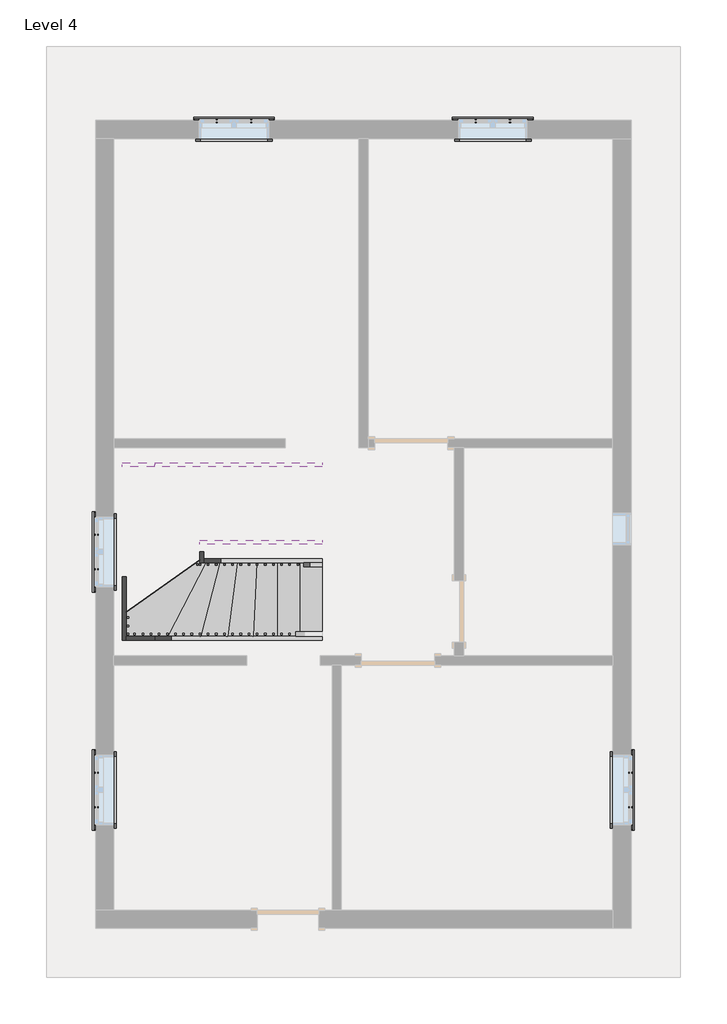
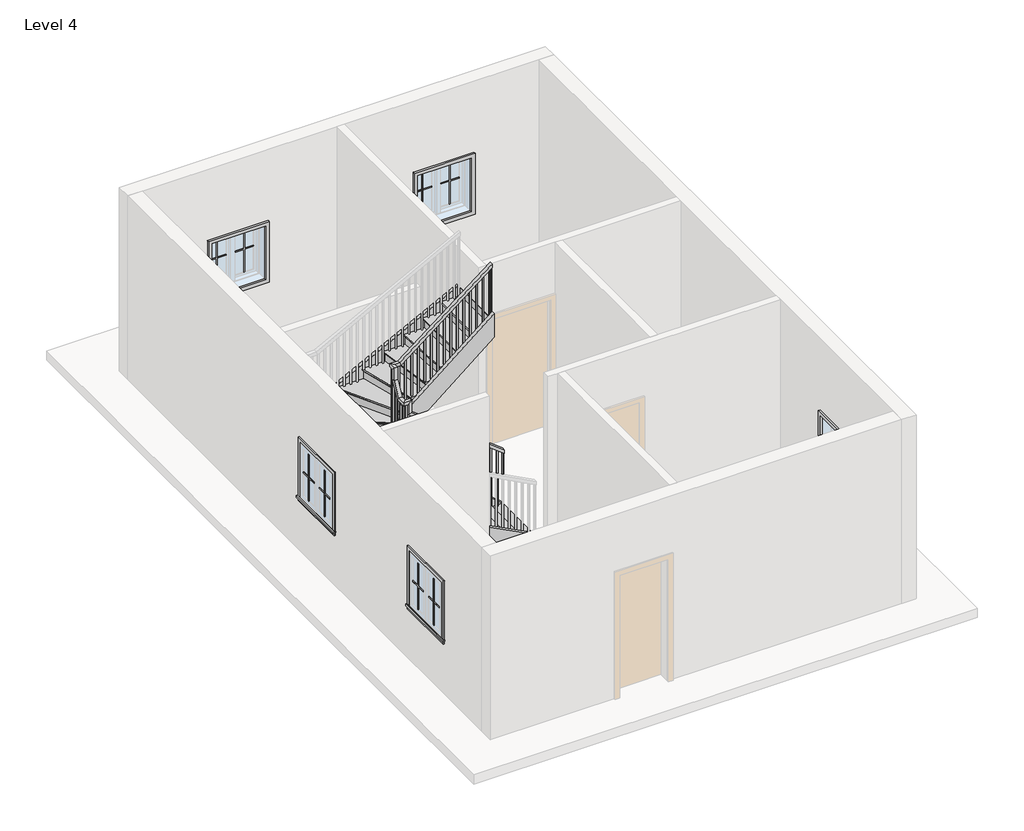
# One storey, part 2 of 2: 20 proxies, 8 members, 1 railing, 1 stair flight.
"""IFC4 building model written with IfcOpenShell, lengths in millimetres."""

from ifc_helpers import new_model, si_unit, frame, origin, place, context, project, spatial, polyline, outline, extrude, faceted_brep, transform, mapped, element, save
from components import muntin_pattern_2x2_muntin_pattern_2x2_b3fe6957, muntin_pattern_2x2_muntin_pattern_2x2_3e0ecaf2, trim_window_exterior_flat_with_sill_41619996, trim_window_interior_flat_picture_frame_51c85655, stair_flight_c61886c8

model = new_model("IFC4")

# Units and contexts
model_context = context("Model", 3, world=origin())
ifc_project = project(units=[si_unit("LENGTHUNIT", "METRE", prefix="MILLI")], contexts=[model_context])

# Site, building, storey
site = spatial("IfcSite", under=ifc_project)
building = spatial("IfcBuilding", under=site)
storey = spatial("IfcBuildingStorey", under=building, Name="Level 4", Elevation=6400.8)

# Proxies
placement = place(None, origin())
muntin_pattern_2x2_muntin_pattern_2x2_shape = muntin_pattern_2x2_muntin_pattern_2x2_b3fe6957(model_context)
element("IfcBuildingElementProxy", 1, Name="Muntin Pattern_2x2 : Muntin Pattern_2x2", ObjectType="Muntin Pattern_2x2 : Muntin Pattern_2x2", at=placement, inside=storey, context=model_context, shape_type="MappedRepresentation", body=[
    mapped(muntin_pattern_2x2_muntin_pattern_2x2_shape, transform((-3096.8324167, 5150.2179147, 7385.05), x_axis=(1.0, 0.0, 0.0), y_axis=(0.0, 1.0, 0.0), z_axis=(0.0, 0.0, 1.0))),
])
element("IfcBuildingElementProxy", 2, Name="Muntin Pattern_2x2 : Muntin Pattern_2x2", ObjectType="Muntin Pattern_2x2 : Muntin Pattern_2x2", at=placement, inside=storey, context=model_context, shape_type="MappedRepresentation", body=[
    mapped(muntin_pattern_2x2_muntin_pattern_2x2_shape, transform((122.6175833, 5150.2179147, 7385.05), x_axis=(1.0, 0.0, 0.0), y_axis=(0.0, 1.0, 0.0), z_axis=(0.0, 0.0, 1.0))),
])
element("IfcBuildingElementProxy", 3, Name="Muntin Pattern_2x2 : Muntin Pattern_2x2", ObjectType="Muntin Pattern_2x2 : Muntin Pattern_2x2", at=placement, inside=storey, context=model_context, shape_type="MappedRepresentation", body=[
    mapped(muntin_pattern_2x2_muntin_pattern_2x2_shape, transform((2051.4300833, -2960.3195853, 7385.05), x_axis=(0.0, -1.0, 0.0), y_axis=(1.0, 0.0, 0.0), z_axis=(0.0, 0.0, 1.0))),
])
element("IfcBuildingElementProxy", 4, Name="Muntin Pattern_2x2 : Muntin Pattern_2x2", ObjectType="Muntin Pattern_2x2 : Muntin Pattern_2x2", at=placement, inside=storey, context=model_context, shape_type="MappedRepresentation", body=[
    mapped(muntin_pattern_2x2_muntin_pattern_2x2_shape, transform((-4597.0199167, -3388.9445853, 7385.05), x_axis=(0.0, 1.0, 0.0), y_axis=(-1.0, 0.0, 0.0), z_axis=(0.0, 0.0, 1.0))),
])
element("IfcBuildingElementProxy", 5, Name="Muntin Pattern_2x2 : Muntin Pattern_2x2", ObjectType="Muntin Pattern_2x2 : Muntin Pattern_2x2", at=placement, inside=storey, context=model_context, shape_type="MappedRepresentation", body=[
    mapped(muntin_pattern_2x2_muntin_pattern_2x2_shape, transform((-4597.0199167, -426.6695853, 7385.05), x_axis=(0.0, 1.0, 0.0), y_axis=(-1.0, 0.0, 0.0), z_axis=(0.0, 0.0, 1.0))),
])
muntin_pattern_2x2_muntin_pattern_2x2_2_shape = muntin_pattern_2x2_muntin_pattern_2x2_3e0ecaf2(model_context)
element("IfcBuildingElementProxy", 6, Name="Muntin Pattern_2x2 : Muntin Pattern_2x2", ObjectType="Muntin Pattern_2x2 : Muntin Pattern_2x2", at=placement, inside=storey, context=model_context, shape_type="MappedRepresentation", body=[
    mapped(muntin_pattern_2x2_muntin_pattern_2x2_2_shape, transform((-2668.2074167, 5150.2179147, 7385.05), x_axis=(-1.0, 0.0, 0.0), y_axis=(0.0, -1.0, 0.0), z_axis=(0.0, 0.0, 1.0))),
])
element("IfcBuildingElementProxy", 7, Name="Muntin Pattern_2x2 : Muntin Pattern_2x2", ObjectType="Muntin Pattern_2x2 : Muntin Pattern_2x2", at=placement, inside=storey, context=model_context, shape_type="MappedRepresentation", body=[
    mapped(muntin_pattern_2x2_muntin_pattern_2x2_2_shape, transform((551.2425833, 5150.2179147, 7385.05), x_axis=(-1.0, 0.0, 0.0), y_axis=(0.0, -1.0, 0.0), z_axis=(0.0, 0.0, 1.0))),
])
element("IfcBuildingElementProxy", 8, Name="Muntin Pattern_2x2 : Muntin Pattern_2x2", ObjectType="Muntin Pattern_2x2 : Muntin Pattern_2x2", at=placement, inside=storey, context=model_context, shape_type="MappedRepresentation", body=[
    mapped(muntin_pattern_2x2_muntin_pattern_2x2_2_shape, transform((2051.4300833, -3388.9445853, 7385.05), x_axis=(0.0, 1.0, 0.0), y_axis=(-1.0, 0.0, 0.0), z_axis=(0.0, 0.0, 1.0))),
])
element("IfcBuildingElementProxy", 9, Name="Muntin Pattern_2x2 : Muntin Pattern_2x2", ObjectType="Muntin Pattern_2x2 : Muntin Pattern_2x2", at=placement, inside=storey, context=model_context, shape_type="MappedRepresentation", body=[
    mapped(muntin_pattern_2x2_muntin_pattern_2x2_2_shape, transform((-4597.0199167, -2960.3195853, 7385.05), x_axis=(0.0, -1.0, 0.0), y_axis=(1.0, 0.0, 0.0), z_axis=(0.0, 0.0, 1.0))),
])
element("IfcBuildingElementProxy", 10, Name="Muntin Pattern_2x2 : Muntin Pattern_2x2", ObjectType="Muntin Pattern_2x2 : Muntin Pattern_2x2", at=placement, inside=storey, context=model_context, shape_type="MappedRepresentation", body=[
    mapped(muntin_pattern_2x2_muntin_pattern_2x2_2_shape, transform((-4597.0199167, 1.9554147, 7385.05), x_axis=(0.0, -1.0, 0.0), y_axis=(1.0, 0.0, 0.0), z_axis=(0.0, 0.0, 1.0))),
])
trim_window_exterior_flat_with_sill_shape = trim_window_exterior_flat_with_sill_41619996(model_context)
element("IfcBuildingElementProxy", 11, Name="Trim-Window-Exterior-Flat : with Sill", ObjectType="Trim-Window-Exterior-Flat : with Sill", at=placement, inside=storey, context=model_context, shape_type="MappedRepresentation", body=[
    mapped(trim_window_exterior_flat_with_sill_shape, transform((-2882.5199167, 5159.7429147, 8229.6), x_axis=(-1.0, 0.0, 0.0), y_axis=(0.0, 0.0, 1.0), z_axis=(0.0, 1.0, 0.0))),
])
element("IfcBuildingElementProxy", 12, Name="Trim-Window-Exterior-Flat : with Sill", ObjectType="Trim-Window-Exterior-Flat : with Sill", at=placement, inside=storey, context=model_context, shape_type="MappedRepresentation", body=[
    mapped(trim_window_exterior_flat_with_sill_shape, transform((336.9300833, 5159.7429147, 8229.6), x_axis=(-1.0, 0.0, 0.0), y_axis=(0.0, 0.0, 1.0), z_axis=(0.0, 1.0, 0.0))),
])
element("IfcBuildingElementProxy", 13, Name="Trim-Window-Exterior-Flat : with Sill", ObjectType="Trim-Window-Exterior-Flat : with Sill", at=placement, inside=storey, context=model_context, shape_type="MappedRepresentation", body=[
    mapped(trim_window_exterior_flat_with_sill_shape, transform((2060.9550833, -3174.6320853, 8229.6), x_axis=(0.0, 1.0, 0.0), y_axis=(0.0, 0.0, 1.0), z_axis=(1.0, 0.0, 0.0))),
])
element("IfcBuildingElementProxy", 14, Name="Trim-Window-Exterior-Flat : with Sill", ObjectType="Trim-Window-Exterior-Flat : with Sill", at=placement, inside=storey, context=model_context, shape_type="MappedRepresentation", body=[
    mapped(trim_window_exterior_flat_with_sill_shape, transform((-4606.5449167, -3174.6320853, 8229.6), x_axis=(0.0, -1.0, 0.0), y_axis=(0.0, 0.0, 1.0), z_axis=(-1.0, 0.0, 0.0))),
])
element("IfcBuildingElementProxy", 15, Name="Trim-Window-Exterior-Flat : with Sill", ObjectType="Trim-Window-Exterior-Flat : with Sill", at=placement, inside=storey, context=model_context, shape_type="MappedRepresentation", body=[
    mapped(trim_window_exterior_flat_with_sill_shape, transform((-4606.5449167, -212.3570853, 8229.6), x_axis=(0.0, -1.0, 0.0), y_axis=(0.0, 0.0, 1.0), z_axis=(-1.0, 0.0, 0.0))),
])
trim_window_interior_flat_picture_frame_shape = trim_window_interior_flat_picture_frame_51c85655(model_context)
element("IfcBuildingElementProxy", 16, Name="Trim-Window-Interior-Flat : Picture Frame", ObjectType="Trim-Window-Interior-Flat : Picture Frame", at=placement, inside=storey, context=model_context, shape_type="MappedRepresentation", body=[
    mapped(trim_window_interior_flat_picture_frame_shape, transform((-2882.5199167, 4931.1429147, 8229.6), x_axis=(1.0, 0.0, 0.0), y_axis=(0.0, 0.0, 1.0), z_axis=(0.0, -1.0, 0.0))),
])
element("IfcBuildingElementProxy", 17, Name="Trim-Window-Interior-Flat : Picture Frame", ObjectType="Trim-Window-Interior-Flat : Picture Frame", at=placement, inside=storey, context=model_context, shape_type="MappedRepresentation", body=[
    mapped(trim_window_interior_flat_picture_frame_shape, transform((336.9300833, 4931.1429147, 8229.6), x_axis=(1.0, 0.0, 0.0), y_axis=(0.0, 0.0, 1.0), z_axis=(0.0, -1.0, 0.0))),
])
element("IfcBuildingElementProxy", 18, Name="Trim-Window-Interior-Flat : Picture Frame", ObjectType="Trim-Window-Interior-Flat : Picture Frame", at=placement, inside=storey, context=model_context, shape_type="MappedRepresentation", body=[
    mapped(trim_window_interior_flat_picture_frame_shape, transform((1832.3550833, -3174.6320853, 8229.6), x_axis=(0.0, -1.0, 0.0), y_axis=(0.0, 0.0, 1.0), z_axis=(-1.0, 0.0, 0.0))),
])
element("IfcBuildingElementProxy", 19, Name="Trim-Window-Interior-Flat : Picture Frame", ObjectType="Trim-Window-Interior-Flat : Picture Frame", at=placement, inside=storey, context=model_context, shape_type="MappedRepresentation", body=[
    mapped(trim_window_interior_flat_picture_frame_shape, transform((-4377.9449167, -3174.6320853, 8229.6), x_axis=(0.0, 1.0, 0.0), y_axis=(0.0, 0.0, 1.0), z_axis=(1.0, 0.0, 0.0))),
])
element("IfcBuildingElementProxy", 20, Name="Trim-Window-Interior-Flat : Picture Frame", ObjectType="Trim-Window-Interior-Flat : Picture Frame", at=placement, inside=storey, context=model_context, shape_type="MappedRepresentation", body=[
    mapped(trim_window_interior_flat_picture_frame_shape, transform((-4377.9449167, -212.3570853, 8229.6), x_axis=(0.0, 1.0, 0.0), y_axis=(0.0, 0.0, 1.0), z_axis=(1.0, 0.0, 0.0))),
])

# Members
element("IfcMember", 21, ObjectType="Stringer - 2\" Width", at=placement, inside=storey, context=model_context, shape_type="SweptSolid", body=[
    extrude(outline(polyline([(6400.8, -1783.4132248), (6630.439954, -1783.4132248), (7706.1956453, -3870.8304165), (7363.300629, -3870.8304165), (6400.8, -2003.1755424), (6400.8, -1783.4132248)])), frame((0.0, -1310.9070853, 0.0), z_axis=(0.0, 1.0, 0.0), x_axis=(0.0, 0.0, 1.0)), (0.0, 0.0, 1.0), 50.8),
])
element("IfcMember", 22, ObjectType="Stringer - 2\" Width", at=placement, inside=storey, context=model_context, shape_type="SweptSolid", body=[
    extrude(outline(polyline([(-3870.8304165, -1260.1070853), (-3870.8304165, -1310.9070853), (-4225.5449167, -1310.9070853), (-4225.5449167, -1260.1070853), (-3870.8304165, -1260.1070853)])), frame((0.0, 0.0, 7363.300629), z_axis=(0.0, 0.0, 1.0), x_axis=(1.0, 0.0, 0.0)), (0.0, 0.0, 1.0), 342.8950162),
])
element("IfcMember", 23, ObjectType="Stringer - 2\" Width", at=placement, inside=storey, context=model_context, shape_type="SweptSolid", body=[
    extrude(outline(polyline([(-1310.9070853, 7401.3956453), (-1310.9070853, 7689.8952212), (811.1127974, 8370.7972697), (848.0929147, 8370.7972697), (848.0929147, 8039.7682298), (-1141.3846024, 7401.3956453), (-1310.9070853, 7401.3956453)])), frame((-4276.3449167, 0.0, 0.0), z_axis=(1.0, 0.0, 0.0), x_axis=(0.0, 1.0, 0.0)), (0.0, 0.0, 1.0), 50.8),
])
element("IfcMember", 24, ObjectType="Stringer - 2\" Width", at=placement, inside=storey, context=model_context, shape_type="SweptSolid", body=[
    extrude(outline(polyline([(-4276.3449167, 848.0929147), (-4276.3449167, 898.8929147), (-3870.8304165, 898.8929147), (-3870.8304165, 848.0929147), (-4276.3449167, 848.0929147)])), frame((0.0, 0.0, 8050.6904473), z_axis=(0.0, 0.0, 1.0), x_axis=(1.0, 0.0, 0.0)), (0.0, 0.0, 1.0), 320.1068224),
])
element("IfcMember", 25, ObjectType="Stringer - 2\" Width", at=placement, inside=storey, context=model_context, shape_type="SweptSolid", body=[
    extrude(outline(polyline([(8370.7972697, -3870.8304165), (8050.6904473, -3870.8304165), (9126.4461385, -1783.4132248), (9446.5529609, -1783.4132248), (8370.7972697, -3870.8304165)])), frame((0.0, 848.0929147, 0.0), z_axis=(0.0, 1.0, 0.0), x_axis=(0.0, 0.0, 1.0)), (0.0, 0.0, 1.0), 50.8),
])
element("IfcMember", 26, ObjectType="Stringer - 2\" Width", at=placement, inside=storey, context=model_context, shape_type="SweptSolid", body=[
    extrude(outline(polyline([(6400.8, -1783.4132248), (6576.9764461, -1783.4132248), (7781.218648, -3260.3449167), (7387.9410923, -3260.3449167), (6400.8, -2049.6748694), (6400.8, -1783.4132248)])), frame((0.0, -345.7070853, 0.0), z_axis=(0.0, 1.0, 0.0), x_axis=(0.0, 0.0, 1.0)), (0.0, 0.0, 1.0), 50.8),
])
element("IfcMember", 27, ObjectType="Stringer - 2\" Width", at=placement, inside=storey, context=model_context, shape_type="SweptSolid", body=[
    extrude(outline(polyline([(-345.7070853, 7429.3617647), (-345.7070853, 7974.0682978), (-139.0699679, 8326.9409689), (-117.1070853, 8326.9409689), (-117.1070853, 7761.265107), (-311.464868, 7429.3617647), (-345.7070853, 7429.3617647)])), frame((-3311.1449167, 0.0, 0.0), z_axis=(1.0, 0.0, 0.0), x_axis=(0.0, 1.0, 0.0)), (0.0, 0.0, 1.0), 50.8),
])
element("IfcMember", 28, ObjectType="Stringer - 2\" Width", at=placement, inside=storey, context=model_context, shape_type="SweptSolid", body=[
    extrude(outline(polyline([(8326.9409689, -3311.1449167), (7933.6634131, -3311.1449167), (9179.3262875, -1783.4132248), (9572.6038432, -1783.4132248), (8326.9409689, -3311.1449167)])), frame((0.0, -117.1070853, 0.0), z_axis=(0.0, 1.0, 0.0), x_axis=(0.0, 0.0, 1.0)), (0.0, 0.0, 1.0), 50.8),
])

# Railing
element("IfcRailing", 29, ObjectType="Handrail - Rectangular", at=placement, inside=storey, context=model_context, shape_type="SolidModel", body=[
    faceted_brep([(-1783.4132248, -396.5070853, 7484.5333333), (-1783.4132248, -396.5070853, 7420.2000346), (-1783.4132248, -345.7070853, 7420.2000346), (-1783.4132248, -345.7070853, 7484.5333333), (-3234.9449167, -396.5070853, 8612.4191036), (-3285.7449167, -396.5070853, 8587.5590024), (-3285.7449167, -345.7070853, 8587.5590024), (-3234.9449167, -345.7070853, 8612.4191036), (-3234.9449167, -396.5070853, 8815.4281882), (-3285.7449167, -396.5070853, 8764.6281882), (-3285.7449167, -345.7070853, 8764.6281882), (-3234.9449167, -345.7070853, 8815.4281882), (-3361.9449167, -396.5070853, 8815.4281882), (-3361.9449167, -396.5070853, 8764.6281882), (-3311.1449167, -345.7070853, 8764.6281882), (-3311.1449167, -345.7070853, 8815.4281882), (-3361.9449167, -269.5070853, 8815.4281882), (-3361.9449167, -240.3857515, 8764.6281882), (-3311.1449167, -240.3857515, 8764.6281882), (-3311.1449167, -269.5070853, 8815.4281882), (-3361.9449167, -142.5070853, 9032.3051451), (-3361.9449167, -91.7070853, 9018.5256424), (-3311.1449167, -91.7070853, 9018.5256424), (-3311.1449167, -142.5070853, 9032.3051451), (-3361.9449167, -142.5070853, 9235.3142297), (-3361.9449167, -91.7070853, 9184.5142297), (-3311.1449167, -91.7070853, 9184.5142297), (-3311.1449167, -142.5070853, 9235.3142297), (-3361.9449167, -15.5070853, 9235.3142297), (-3361.9449167, -15.5070853, 9184.5142297), (-3311.1449167, -66.3070853, 9184.5142297), (-3311.1449167, -66.3070853, 9235.3142297), (-3234.9449167, -15.5070853, 9235.3142297), (-3217.5282487, -15.5070853, 9184.5142297), (-3217.5282487, -66.3070853, 9184.5142297), (-3234.9449167, -66.3070853, 9235.3142297), (-1783.4132248, -15.5070853, 10363.2), (-1783.4132248, -66.3070853, 10363.2), (-1783.4132248, -66.3070853, 10298.8667013), (-1783.4132248, -15.5070853, 10298.8667013)], [[[0, 1, 2, 3]], [[1, 0, 4, 5]], [[2, 1, 5, 6]], [[3, 2, 6, 7]], [[0, 3, 7, 4]], [[5, 4, 8, 9]], [[6, 5, 9, 10]], [[7, 6, 10, 11]], [[4, 7, 11, 8]], [[9, 8, 12, 13]], [[10, 9, 13, 14]], [[11, 10, 14, 15]], [[8, 11, 15, 12]], [[13, 12, 16, 17]], [[14, 13, 17, 18]], [[15, 14, 18, 19]], [[12, 15, 19, 16]], [[17, 16, 20, 21]], [[18, 17, 21, 22]], [[19, 18, 22, 23]], [[16, 19, 23, 20]], [[21, 20, 24, 25]], [[22, 21, 25, 26]], [[23, 22, 26, 27]], [[20, 23, 27, 24]], [[25, 24, 28, 29]], [[26, 25, 29, 30]], [[27, 26, 30, 31]], [[24, 27, 31, 28]], [[29, 28, 32, 33]], [[30, 29, 33, 34]], [[31, 30, 34, 35]], [[28, 31, 35, 32]], [[36, 37, 38, 39]], [[33, 32, 36, 39]], [[34, 33, 39, 38]], [[35, 34, 38, 37]], [[32, 35, 37, 36]]]),
    extrude(outline(polyline([(10283.6316852, -1803.0199167), (10268.8292361, -1822.0699167), (9279.4666667, -1822.0699167), (9279.4666667, -1803.0199167), (10283.6316852, -1803.0199167)])), frame((0.0, -50.4320853, 0.0), z_axis=(0.0, 1.0, 0.0), x_axis=(0.0, 0.0, 1.0)), (0.0, 0.0, 1.0), 19.05),
    extrude(outline(polyline([(10204.6852902, -1904.6199167), (10189.8828411, -1923.6699167), (9279.4666667, -1923.6699167), (9279.4666667, -1904.6199167), (10204.6852902, -1904.6199167)])), frame((0.0, -50.4320853, 0.0), z_axis=(0.0, 1.0, 0.0), x_axis=(0.0, 0.0, 1.0)), (0.0, 0.0, 1.0), 19.05),
    extrude(outline(polyline([(10125.7388952, -2006.2199167), (10110.9364462, -2025.2699167), (9279.4666667, -2025.2699167), (9279.4666667, -2006.2199167), (10125.7388952, -2006.2199167)])), frame((0.0, -50.4320853, 0.0), z_axis=(0.0, 1.0, 0.0), x_axis=(0.0, 0.0, 1.0)), (0.0, 0.0, 1.0), 19.05),
    extrude(outline(polyline([(10046.7925003, -2107.8199167), (10031.9900512, -2126.8699167), (9110.1333333, -2126.8699167), (9110.1333333, -2107.8199167), (10046.7925003, -2107.8199167)])), frame((0.0, -50.4320853, 0.0), z_axis=(0.0, 1.0, 0.0), x_axis=(0.0, 0.0, 1.0)), (0.0, 0.0, 1.0), 19.05),
    extrude(outline(polyline([(9967.8461053, -2209.4199167), (9953.0436562, -2228.4699167), (9110.1333333, -2228.4699167), (9110.1333333, -2209.4199167), (9967.8461053, -2209.4199167)])), frame((0.0, -50.4320853, 0.0), z_axis=(0.0, 1.0, 0.0), x_axis=(0.0, 0.0, 1.0)), (0.0, 0.0, 1.0), 19.05),
    extrude(outline(polyline([(9888.8997103, -2311.0199167), (9874.0972613, -2330.0699167), (9110.1333333, -2330.0699167), (9110.1333333, -2311.0199167), (9888.8997103, -2311.0199167)])), frame((0.0, -50.4320853, 0.0), z_axis=(0.0, 1.0, 0.0), x_axis=(0.0, 0.0, 1.0)), (0.0, 0.0, 1.0), 19.05),
    extrude(outline(polyline([(9809.9533154, -2412.6199167), (9795.1508663, -2431.6699167), (8940.8, -2431.6699167), (8940.8, -2412.6199167), (9809.9533154, -2412.6199167)])), frame((0.0, -50.4320853, 0.0), z_axis=(0.0, 1.0, 0.0), x_axis=(0.0, 0.0, 1.0)), (0.0, 0.0, 1.0), 19.05),
    extrude(outline(polyline([(9731.0069204, -2514.2199167), (9716.2044713, -2533.2699167), (8940.8, -2533.2699167), (8940.8, -2514.2199167), (9731.0069204, -2514.2199167)])), frame((0.0, -50.4320853, 0.0), z_axis=(0.0, 1.0, 0.0), x_axis=(0.0, 0.0, 1.0)), (0.0, 0.0, 1.0), 19.05),
    extrude(outline(polyline([(9652.0605254, -2615.8199167), (9637.2580764, -2634.8699167), (8771.4666667, -2634.8699167), (8771.4666667, -2615.8199167), (9652.0605254, -2615.8199167)])), frame((0.0, -50.4320853, 0.0), z_axis=(0.0, 1.0, 0.0), x_axis=(0.0, 0.0, 1.0)), (0.0, 0.0, 1.0), 19.05),
    extrude(outline(polyline([(9573.1141304, -2717.4199167), (9558.3116814, -2736.4699167), (8771.4666667, -2736.4699167), (8771.4666667, -2717.4199167), (9573.1141304, -2717.4199167)])), frame((0.0, -50.4320853, 0.0), z_axis=(0.0, 1.0, 0.0), x_axis=(0.0, 0.0, 1.0)), (0.0, 0.0, 1.0), 19.05),
    extrude(outline(polyline([(9494.1677355, -2819.0199167), (9479.3652864, -2838.0699167), (8771.4666667, -2838.0699167), (8771.4666667, -2819.0199167), (9494.1677355, -2819.0199167)])), frame((0.0, -50.4320853, 0.0), z_axis=(0.0, 1.0, 0.0), x_axis=(0.0, 0.0, 1.0)), (0.0, 0.0, 1.0), 19.05),
    extrude(outline(polyline([(9415.2213405, -2920.6199167), (9400.4188914, -2939.6699167), (8602.1333333, -2939.6699167), (8602.1333333, -2920.6199167), (9415.2213405, -2920.6199167)])), frame((0.0, -50.4320853, 0.0), z_axis=(0.0, 1.0, 0.0), x_axis=(0.0, 0.0, 1.0)), (0.0, 0.0, 1.0), 19.05),
    extrude(outline(polyline([(9336.2749455, -3022.2199167), (9321.4724965, -3041.2699167), (8602.1333333, -3041.2699167), (8602.1333333, -3022.2199167), (9336.2749455, -3022.2199167)])), frame((0.0, -50.4320853, 0.0), z_axis=(0.0, 1.0, 0.0), x_axis=(0.0, 0.0, 1.0)), (0.0, 0.0, 1.0), 19.05),
    extrude(outline(polyline([(9257.3285506, -3123.8199167), (9242.5261015, -3142.8699167), (8432.8, -3142.8699167), (8432.8, -3123.8199167), (9257.3285506, -3123.8199167)])), frame((0.0, -50.4320853, 0.0), z_axis=(0.0, 1.0, 0.0), x_axis=(0.0, 0.0, 1.0)), (0.0, 0.0, 1.0), 19.05),
    extrude(outline(polyline([(9178.3821556, -3225.4199167), (9163.5797065, -3244.4699167), (8432.8, -3244.4699167), (8432.8, -3225.4199167), (9178.3821556, -3225.4199167)])), frame((0.0, -50.4320853, 0.0), z_axis=(0.0, 1.0, 0.0), x_axis=(0.0, 0.0, 1.0)), (0.0, 0.0, 1.0), 19.05),
    extrude(outline(polyline([(-3327.0199167, -75.8320853), (-3346.0699167, -75.8320853), (-3346.0699167, -56.7820853), (-3327.0199167, -56.7820853), (-3327.0199167, -75.8320853)])), frame((0.0, 0.0, 8094.1333333), z_axis=(0.0, 0.0, 1.0), x_axis=(1.0, 0.0, 0.0)), (0.0, 0.0, 1.0), 1090.3808964),
    extrude(outline(polyline([(-177.4320853, 8872.1336964), (-158.3820853, 8904.66524), (-158.3820853, 7924.8), (-177.4320853, 7924.8), (-177.4320853, 8872.1336964)])), frame((-3346.0699167, 0.0, 0.0), z_axis=(1.0, 0.0, 0.0), x_axis=(0.0, 1.0, 0.0)), (0.0, 0.0, 1.0), 19.05),
    extrude(outline(polyline([(-279.0320853, 8698.6321309), (-259.9820853, 8731.1636744), (-259.9820853, 7755.4666667), (-279.0320853, 7755.4666667), (-279.0320853, 8698.6321309)])), frame((-3346.0699167, 0.0, 0.0), z_axis=(1.0, 0.0, 0.0), x_axis=(0.0, 1.0, 0.0)), (0.0, 0.0, 1.0), 19.05),
    extrude(outline(polyline([(-3297.8882248, -361.5820853), (-3297.8882248, -380.6320853), (-3316.9382248, -380.6320853), (-3316.9382248, -361.5820853), (-3297.8882248, -361.5820853)])), frame((0.0, 0.0, 7586.1333333), z_axis=(0.0, 0.0, 1.0), x_axis=(1.0, 0.0, 0.0)), (0.0, 0.0, 1.0), 1178.4948549),
    extrude(outline(polyline([(8518.0483397, -3196.2882248), (8532.8507888, -3215.3382248), (7416.8, -3215.3382248), (7416.8, -3196.2882248), (8518.0483397, -3196.2882248)])), frame((0.0, -380.6320853, 0.0), z_axis=(0.0, 1.0, 0.0), x_axis=(0.0, 0.0, 1.0)), (0.0, 0.0, 1.0), 19.05),
    extrude(outline(polyline([(8439.1019447, -3094.6882248), (8453.9043938, -3113.7382248), (7416.8, -3113.7382248), (7416.8, -3094.6882248), (8439.1019447, -3094.6882248)])), frame((0.0, -380.6320853, 0.0), z_axis=(0.0, 1.0, 0.0), x_axis=(0.0, 0.0, 1.0)), (0.0, 0.0, 1.0), 19.05),
    extrude(outline(polyline([(8360.1555498, -2993.0882248), (8374.9579988, -3012.1382248), (7247.4666667, -3012.1382248), (7247.4666667, -2993.0882248), (8360.1555498, -2993.0882248)])), frame((0.0, -380.6320853, 0.0), z_axis=(0.0, 1.0, 0.0), x_axis=(0.0, 0.0, 1.0)), (0.0, 0.0, 1.0), 19.05),
    extrude(outline(polyline([(8281.2091548, -2891.4882248), (8296.0116039, -2910.5382248), (7247.4666667, -2910.5382248), (7247.4666667, -2891.4882248), (8281.2091548, -2891.4882248)])), frame((0.0, -380.6320853, 0.0), z_axis=(0.0, 1.0, 0.0), x_axis=(0.0, 0.0, 1.0)), (0.0, 0.0, 1.0), 19.05),
    extrude(outline(polyline([(8202.2627598, -2789.8882248), (8217.0652089, -2808.9382248), (7078.1333333, -2808.9382248), (7078.1333333, -2789.8882248), (8202.2627598, -2789.8882248)])), frame((0.0, -380.6320853, 0.0), z_axis=(0.0, 1.0, 0.0), x_axis=(0.0, 0.0, 1.0)), (0.0, 0.0, 1.0), 19.05),
    extrude(outline(polyline([(8123.3163649, -2688.2882248), (8138.1188139, -2707.3382248), (7078.1333333, -2707.3382248), (7078.1333333, -2688.2882248), (8123.3163649, -2688.2882248)])), frame((0.0, -380.6320853, 0.0), z_axis=(0.0, 1.0, 0.0), x_axis=(0.0, 0.0, 1.0)), (0.0, 0.0, 1.0), 19.05),
    extrude(outline(polyline([(8044.3699699, -2586.6882248), (8059.1724189, -2605.7382248), (6908.8, -2605.7382248), (6908.8, -2586.6882248), (8044.3699699, -2586.6882248)])), frame((0.0, -380.6320853, 0.0), z_axis=(0.0, 1.0, 0.0), x_axis=(0.0, 0.0, 1.0)), (0.0, 0.0, 1.0), 19.05),
    extrude(outline(polyline([(7965.4235749, -2485.0882248), (7980.226024, -2504.1382248), (6908.8, -2504.1382248), (6908.8, -2485.0882248), (7965.4235749, -2485.0882248)])), frame((0.0, -380.6320853, 0.0), z_axis=(0.0, 1.0, 0.0), x_axis=(0.0, 0.0, 1.0)), (0.0, 0.0, 1.0), 19.05),
    extrude(outline(polyline([(7886.4771799, -2383.4882248), (7901.279629, -2402.5382248), (6908.8, -2402.5382248), (6908.8, -2383.4882248), (7886.4771799, -2383.4882248)])), frame((0.0, -380.6320853, 0.0), z_axis=(0.0, 1.0, 0.0), x_axis=(0.0, 0.0, 1.0)), (0.0, 0.0, 1.0), 19.05),
    extrude(outline(polyline([(7807.530785, -2281.8882248), (7822.333234, -2300.9382248), (6739.4666667, -2300.9382248), (6739.4666667, -2281.8882248), (7807.530785, -2281.8882248)])), frame((0.0, -380.6320853, 0.0), z_axis=(0.0, 1.0, 0.0), x_axis=(0.0, 0.0, 1.0)), (0.0, 0.0, 1.0), 19.05),
    extrude(outline(polyline([(7728.58439, -2180.2882248), (7743.3868391, -2199.3382248), (6739.4666667, -2199.3382248), (6739.4666667, -2180.2882248), (7728.58439, -2180.2882248)])), frame((0.0, -380.6320853, 0.0), z_axis=(0.0, 1.0, 0.0), x_axis=(0.0, 0.0, 1.0)), (0.0, 0.0, 1.0), 19.05),
    extrude(outline(polyline([(7649.637995, -2078.6882248), (7664.4404441, -2097.7382248), (6739.4666667, -2097.7382248), (6739.4666667, -2078.6882248), (7649.637995, -2078.6882248)])), frame((0.0, -380.6320853, 0.0), z_axis=(0.0, 1.0, 0.0), x_axis=(0.0, 0.0, 1.0)), (0.0, 0.0, 1.0), 19.05),
    extrude(outline(polyline([(7570.6916001, -1977.0882248), (7585.4940491, -1996.1382248), (6570.1333333, -1996.1382248), (6570.1333333, -1977.0882248), (7570.6916001, -1977.0882248)])), frame((0.0, -380.6320853, 0.0), z_axis=(0.0, 1.0, 0.0), x_axis=(0.0, 0.0, 1.0)), (0.0, 0.0, 1.0), 19.05),
    extrude(outline(polyline([(7491.7452051, -1875.4882248), (7506.5476541, -1894.5382248), (6570.1333333, -1894.5382248), (6570.1333333, -1875.4882248), (7491.7452051, -1875.4882248)])), frame((0.0, -380.6320853, 0.0), z_axis=(0.0, 1.0, 0.0), x_axis=(0.0, 0.0, 1.0)), (0.0, 0.0, 1.0), 19.05),
    extrude(outline(polyline([(-3327.0199167, -50.4320853), (-3346.0699167, -50.4320853), (-3346.0699167, -31.3820853), (-3327.0199167, -31.3820853), (-3327.0199167, -50.4320853)])), frame((0.0, 0.0, 8263.4666667), z_axis=(0.0, 0.0, 1.0), x_axis=(1.0, 0.0, 0.0)), (0.0, 0.0, 1.0), 921.0475631),
    extrude(outline(polyline([(-3327.0199167, -361.5820853), (-3327.0199167, -380.6320853), (-3346.0699167, -380.6320853), (-3346.0699167, -361.5820853), (-3327.0199167, -361.5820853)])), frame((0.0, 0.0, 7586.1333333), z_axis=(0.0, 0.0, 1.0), x_axis=(1.0, 0.0, 0.0)), (0.0, 0.0, 1.0), 1178.4948549),
    extrude(outline(polyline([(10298.8667013, -1783.4132248), (10284.0642523, -1802.4632248), (9279.4666667, -1802.4632248), (9279.4666667, -1783.4132248), (10298.8667013, -1783.4132248)])), frame((0.0, -50.4320853, 0.0), z_axis=(0.0, 1.0, 0.0), x_axis=(0.0, 0.0, 1.0)), (0.0, 0.0, 1.0), 19.05),
    extrude(outline(polyline([(7420.2000346, -1783.4132248), (7435.0024837, -1802.4632248), (6570.1333333, -1802.4632248), (6570.1333333, -1783.4132248), (7420.2000346, -1783.4132248)])), frame((0.0, -380.6320853, 0.0), z_axis=(0.0, 1.0, 0.0), x_axis=(0.0, 0.0, 1.0)), (0.0, 0.0, 1.0), 19.05),
])

# Stair flight
stair_flight_shape = stair_flight_c61886c8(model_context)
element("IfcStairFlight", 30, ObjectType="2\" Tread 1\" Nosing 1/4\" Riser", at=placement, inside=storey, context=model_context, shape_type="MappedRepresentation", body=[
    mapped(stair_flight_shape, transform((0.0, 0.0, 0.0), x_axis=(1.0, 0.0, 0.0), y_axis=(0.0, 1.0, 0.0), z_axis=(0.0, 0.0, 1.0))),
])

save(model, "model.ifc")

# Revit data of these elements
# Type "Muntin Pattern_2x2 : Muntin Pattern_2x2"
#   Width [instance default] = 4' - 0"
#   Thickness = 0' - 0 1/2"
#   Height [instance default] = 4' - 0"
#   Distance = 0' - 0 3/4"
#   Interior Material [instance default] = none
#   Exterior Material [instance default] = none
#   Default Elevation = 0
# Type "Trim-Window-Exterior-Flat : with Sill"
#   Trim Width = 0' - 2 1/4"
#   Trim Thickness_Picture Frame = 0' - 1 1/4"
#   Trim Thickness_with Sill = 0' - 0 3/4"
#   Sill Thickness = 0' - 1 1/4"
#   Opening Width [instance default] = 2' - 0"
#   Opening Height [instance default] = 3' - 0"
#   Default Elevation = 4' - 0"
#   Sill = yes
#   Picture Frame = no
#   Trim Material [instance default] = none
# Type "Trim-Window-Interior-Flat : Picture Frame"
#   Trim Thickness_Picture Frame = 0' - 1 1/4"
#   Trim Width = 0' - 2 1/4"
#   Trim Thickness_with Sill = 0' - 0 3/4"
#   Sill Thickness = 0' - 1 1/4"
#   Opening Width [instance default] = 2' - 0"
#   Opening Height [instance default] = 3' - 0"
#   Default Elevation = 4' - 0"
#   Sill = no
#   Picture Frame = yes
#   Trim Material [instance default] = none
# Type "Handrail - Rectangular"
#   Assembly Code = "C2010400"
#   built-in parameter 1008612 = 0.0416667 (stored number, unit not read)
#   built-in parameter 1008611 = 0.0416667 (stored number, unit not read)
#   built-in parameter 1008609 = 0.333333 (stored number, unit not read)
#   built-in parameter 1008604 = 0.166667 (stored number, unit not read)
#   built-in parameter 1008603 = 0.166667 (stored number, unit not read)
#   Railing Height = 3' - 0"
#   built-in parameter 1008630 = 2
#   built-in parameter 1008610 = 2
#   built-in parameter 1008618 = Baluster - Square : 3/4"
# Elements 1, 2, 3, 4, 5, 6, 7, 8, 9, 10 (IfcBuildingElementProxy, "Muntin Pattern_2x2 : Muntin Pattern_2x2")
#   Width = 0' - 11 5/8"
#   Height = 2' - 6 1/2"
#   Interior Material = Wood - Stained
#   Exterior Material = Clad - White
#   Phase Created = New Construction
#   Materials on its faces: "Clad - White", "Wood - Stained"
# Elements 11, 12, 13, 14, 15 (IfcBuildingElementProxy, "Trim-Window-Exterior-Flat : with Sill")
#   Opening Width = 2' - 10"
#   Opening Height = 3' - 0"
#   Trim Material = Clad - White
#   Phase Created = New Construction
#   Materials on its faces: "Clad - White"
# Elements 16, 17, 18, 19, 20 (IfcBuildingElementProxy, "Trim-Window-Interior-Flat : Picture Frame")
#   Opening Width = 2' - 10"
#   Opening Height = 3' - 0"
#   Trim Material = Wood - Stained
#   Phase Created = New Construction
#   Materials on its faces: "Wood - Stained"
# Elements 21, 22, 23, 24, 25, 26, 27, 28 (IfcMember, "Stringer - 2\" Width")
#   Phase Created = New Construction
# Element 29 (IfcRailing, "Handrail - Rectangular")
#   Phase Created = New Construction
# Element 30 (IfcStairFlight, "2\" Tread 1\" Nosing 1/4\" Riser")
#   Phase Created = New Construction
# Materials
#   "Clad - White": class "Wood", colour RGB 242 242 238, transparency 0, Cost = 0
#   "Wood - Stained": class "Wood", colour RGB 224 178 126, transparency 0, Cost = 0
